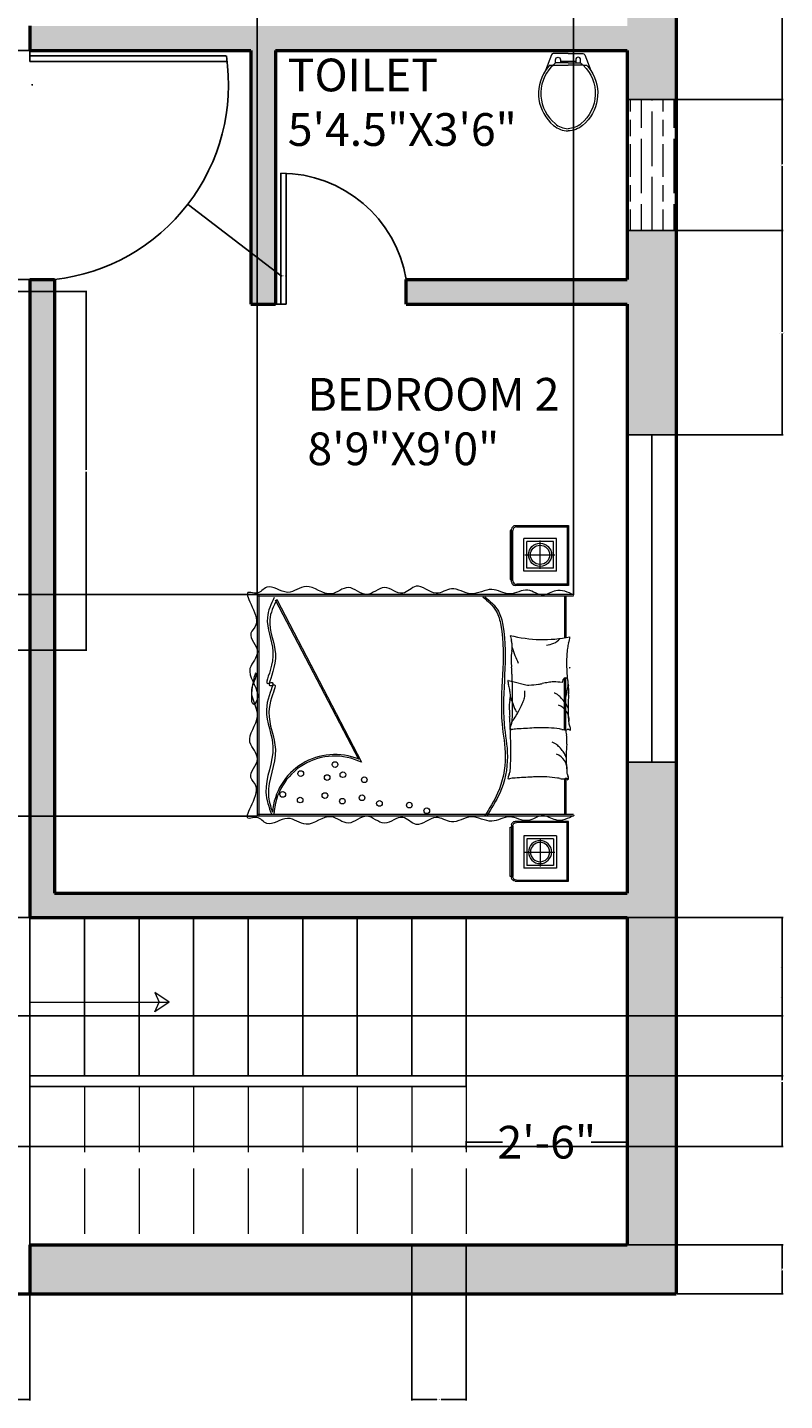
# Model space of a CAD drawing. Units: inches. Extents: x -2 to 282, y -370 to 35.
# Tile 3 of 5: x 143 to 282, y -370 to -119. Entities that reach past the tile are written whole.
import ezdxf

# ---------------------------------------------------------------- set-up
doc = ezdxf.new("R2010")
doc.units = ezdxf.units.IN
doc.header["$MEASUREMENT"] = 0
doc.linetypes.add('ACAD_ISO02W100', pattern=[15, 12, -3])
for name, color, linetype, lineweight in [('A-ANNO-DIMS', 2, 'Continuous', 18), ('A-ANNO-SYMB', 7, 'Continuous', 18), ('A-AREA-IDEN', 7, 'Continuous', 25), ('A-DOOR', 3, 'Continuous', 25), ('A-FLOR-FIXT', 9, 'Continuous', 18), ('A-FLOR-STRS', 7, 'Continuous', 25), ('A-FLOR-STRS-OVHD', 8, 'ACAD_ISO02W100', 18), ('A-FURN', 8, 'Continuous', 18), ('A-GLAZ', 4, 'Continuous', 25), ('A-GLAZ-PATT', 9, 'Continuous', 13), ('A-WALL', 7, 'Continuous', 50), ('A-WALL-PATT', 252, 'Continuous', 13)]:
    doc.layers.add(name, color=color, linetype=linetype, lineweight=lineweight)
doc.styles.get("Standard").update_dxf_attribs({"font": 'arial.ttf'})
doc.dimstyles.get("Standard").update_dxf_attribs({"dimtxt": 0.18, "dimasz": 0.18, "dimexe": 0.18, "dimexo": 0.0625, "dimgap": 0.09, "dimtad": 0, "dimtih": 1, "dimtoh": 1, "dimdec": 0, "dimzin": 0, "dimdsep": 46, "dimlunit": 3, "dimtxsty": 'Standard', "dimcen": 0.09, "dimadec": 0, "dimazin": 0, "dimtfac": 1, "dimtdec": 0, "dimtofl": 0, "dimtmove": 0, "dimatfit": 3, "dimfxl": 1, "dimtolj": 1, "dimtzin": 0, "dimarcsym": 0})

# ---------------------------------------------------------------- blocks, each defined once
blk = doc.blocks.new('*D1')
at = {"layer": 'A-ANNO-DIMS', "color": 0, "lineweight": -2, "transparency": 16777216}
for p, q in [((223.91, -324.22), (223.91, -322.81)), ((224.09, -322.99), (230.55, -322.99)), ((253.23, -322.99), (246.78, -322.99)), ((253.41, -324.22), (253.41, -322.81))]:
    blk.add_line(p, q, dxfattribs=at)
at = {"layer": 'A-ANNO-DIMS', "color": 0, "transparency": 16777216}
for points in [[(224.09, -322.96), (224.09, -323.02), (223.91, -322.99)], [(253.23, -322.96), (253.23, -323.02), (253.41, -322.99)]]:
    blk.add_solid(points, dxfattribs=at)
at = {"layer": 'Defpoints', "color": 0, "transparency": 16777216}
for p in [(223.91, -324.28), (253.41, -322.99), (253.41, -324.28)]:
    blk.add_point(p, dxfattribs=at)
at = {"layer": 'A-ANNO-DIMS', "color": 0, "transparency": 16777216, "insert": (238.66, -322.99), "char_height": 6, "attachment_point": 5}
blk.add_mtext('\\A1;2\'-6"', dxfattribs=at)
blk = doc.blocks.new('WINDOW-60IN')
for p, q in [((0, 0), (0, 60)), ((0, 60), (9, 60)), ((4.5, 60), (4.5, 0)), ((9, 60), (9, 0)), ((9, 0), (0, 0))]:
    blk.add_line(p, q)
blk = doc.blocks.new('DOOR-SWING-24IN')
for p, q in [((24, 2), (0, 2)), ((24, 1), (0, 1)), ((24, 0), (24, 2))]:
    blk.add_line(p, q)
blk.add_arc((23.32, 1), 23.31, 99.4157, 180)
blk = doc.blocks.new('WC-PLAN')
for p, q in [((2.03, 12.04), (2.63, 12.04)), ((2.63, 12.04), (5.42, 12.04)), ((8.21, 12.04), (5.42, 12.04)), ((8.21, 12.04), (8.81, 12.04))]:
    blk.add_line(p, q)
for points in [[(5.42, 14.19), (2.71, 14.19, 0.31031), (2.38, 13.97), (1.26, 11.07, 0.209071)], [(3.12, 12.47), (3.12, 13.07, -1), (4.02, 13.07), (4.02, 12.76)], [(5.42, 14.19), (8.13, 14.19, -0.31031), (8.46, 13.97), (9.58, 11.07, -0.209071)], [(7.72, 12.47), (7.72, 13.07, 1), (6.82, 13.07), (6.82, 12.76)], [(1.26, 11.07, 0.383919), (2.75, 1.02, 0.163732), (5.42, 0, 0.359733)], [(2.34, 11.76, 0.431639), (3.02, 1.35, 0.162618), (5.42, 0.42, 0.470877)], [(2.03, 12.04, 0.040937), (1.26, 11.07, 0.163732)], [(2.63, 12.04, 0.014165), (2.34, 11.76, 0.162618)], [(3.12, 12.47, 0.022712), (2.63, 12.04, 0.162618)], [(5.42, 12.47), (3.12, 12.47, 0.022712)], [(5.42, 12.47), (7.72, 12.47, -0.476108)], [(8.21, 12.04, -0.448546), (7.82, 1.35, -0.162618), (5.42, 0.42, -0.470877)], [(9.58, 11.07, -0.383919), (8.09, 1.02, -0.163732), (5.42, 0, -0.359733)], [(7.72, 12.47, -0.022712), (8.21, 12.04, -0.162618)], [(8.81, 12.04, -0.040937), (9.58, 11.07, -0.163732)]]:
    blk.add_lwpolyline(points, format="xyb")
for points in [[(6.82, 12.76), (4.02, 12.76)], [(4.02, 12.76), (4.02, 12.47)], [(6.82, 12.76), (6.82, 12.47)]]:
    blk.add_lwpolyline(points)
blk = doc.blocks.new('BEDSIDE-TABLE')
for p, q in [((0, 0.94), (0, 10.72)), ((0, 10.72), (11.02, 10.72)), ((0, 10.5), (11.02, 10.5)), ((0.22, 1.16), (0.22, 10.72)), ((10.8, 10.72), (10.8, 1.16)), ((11.02, 10.72), (11.02, 0.94)), ((2.39, 8.51), (2.39, 2.55)), ((8.35, 8.51), (2.39, 8.51)), ((2.92, 7.98), (2.92, 3.08)), ((7.82, 7.98), (2.92, 7.98)), ((5.37, 2.73), (5.37, 8.22)), ((7.82, 7.98), (7.82, 3.08)), ((8.35, 8.51), (8.35, 2.55)), ((7.94, 5.51), (2.73, 5.51)), ((8.35, 2.55), (2.39, 2.55)), ((7.82, 3.08), (2.92, 3.08)), ((10.37, 0.28), (0.66, 0.28)), ((10.15, 0.5), (0.87, 0.5))]:
    blk.add_line(p, q)
blk.add_lwpolyline([(9.94, 0.26), (0.88, 0.26), (0.88, 0), (9.94, 0)], close=True)
for radius in [2.13, 1.77]:
    blk.add_circle((5.37, 5.51), radius)
for centre, start, end in [((0.66, 0.94), 180, 270), ((0.87, 1.16), 180, 270), ((10.15, 1.16), 270, 0), ((10.37, 0.94), 270, 0)]:
    blk.add_arc(centre, 0.655, start, end)
blk = doc.blocks.new('*D26')
at = {"layer": 'A-ANNO-DIMS', "color": 0, "lineweight": -2, "transparency": 16777216}
for p, q in [((262.48, -89.06), (281.97, -89.06)), ((281.79, -89.24), (281.79, -110.25)), ((281.79, -131.63), (281.79, -110.62)), ((262.48, -131.81), (281.97, -131.81))]:
    blk.add_line(p, q, dxfattribs=at)
at = {"layer": 'A-ANNO-DIMS', "color": 0, "transparency": 16777216}
for points in [[(281.76, -89.24), (281.82, -89.24), (281.79, -89.06)], [(281.76, -131.63), (281.82, -131.63), (281.79, -131.81)]]:
    blk.add_solid(points, dxfattribs=at)
at = {"layer": 'Defpoints', "color": 0, "transparency": 16777216}
for p in [(262.41, -89.06), (262.41, -131.81), (281.79, -131.81)]:
    blk.add_point(p, dxfattribs=at)
at = {"layer": 'A-ANNO-DIMS', "color": 0, "transparency": 16777216, "insert": (281.79, -110.44), "char_height": 0.18, "attachment_point": 5}
blk.add_mtext('\\A1;3\'-7"', dxfattribs=at)
blk = doc.blocks.new('*D27')
at = {"layer": 'A-ANNO-DIMS', "color": 0, "lineweight": -2, "transparency": 16777216}
for p, q in [((262.48, -131.81), (281.97, -131.81)), ((281.79, -131.99), (281.79, -143.63)), ((281.79, -155.63), (281.79, -143.99)), ((262.48, -155.81), (281.97, -155.81))]:
    blk.add_line(p, q, dxfattribs=at)
at = {"layer": 'A-ANNO-DIMS', "color": 0, "transparency": 16777216}
for points in [[(281.76, -131.99), (281.82, -131.99), (281.79, -131.81)], [(281.76, -155.63), (281.82, -155.63), (281.79, -155.81)]]:
    blk.add_solid(points, dxfattribs=at)
at = {"layer": 'Defpoints', "color": 0, "transparency": 16777216}
for p in [(262.41, -131.81), (262.41, -155.81), (281.79, -155.81)]:
    blk.add_point(p, dxfattribs=at)
at = {"layer": 'A-ANNO-DIMS', "color": 0, "transparency": 16777216, "insert": (281.79, -143.81), "char_height": 0.18, "attachment_point": 5}
blk.add_mtext('\\A1;2\'-0"', dxfattribs=at)
blk = doc.blocks.new('*D28')
at = {"layer": 'A-ANNO-DIMS', "color": 0, "lineweight": -2, "transparency": 16777216}
for p, q in [((262.48, -155.81), (281.97, -155.81)), ((281.79, -155.99), (281.79, -174.38)), ((281.79, -193.13), (281.79, -174.74)), ((262.48, -193.31), (281.97, -193.31))]:
    blk.add_line(p, q, dxfattribs=at)
at = {"layer": 'A-ANNO-DIMS', "color": 0, "transparency": 16777216}
for points in [[(281.76, -155.99), (281.82, -155.99), (281.79, -155.81)], [(281.76, -193.13), (281.82, -193.13), (281.79, -193.31)]]:
    blk.add_solid(points, dxfattribs=at)
at = {"layer": 'Defpoints', "color": 0, "transparency": 16777216}
for p in [(262.41, -155.81), (262.41, -193.31), (281.79, -193.31)]:
    blk.add_point(p, dxfattribs=at)
at = {"layer": 'A-ANNO-DIMS', "color": 0, "transparency": 16777216, "insert": (281.79, -174.56), "char_height": 0.18, "attachment_point": 5}
blk.add_mtext('\\A1;3\'-1 1/2"', dxfattribs=at)
blk = doc.blocks.new('*D31')
at = {"layer": 'A-ANNO-DIMS', "color": 0, "lineweight": -2, "transparency": 16777216}
for p, q in [((31.48, -281.81), (281.97, -281.81)), ((281.79, -281.99), (281.79, -290.63)), ((281.79, -299.63), (281.79, -290.99)), ((31.48, -299.81), (281.97, -299.81))]:
    blk.add_line(p, q, dxfattribs=at)
at = {"layer": 'A-ANNO-DIMS', "color": 0, "transparency": 16777216}
for points in [[(281.76, -281.99), (281.82, -281.99), (281.79, -281.81)], [(281.76, -299.63), (281.82, -299.63), (281.79, -299.81)]]:
    blk.add_solid(points, dxfattribs=at)
at = {"layer": 'Defpoints', "color": 0, "transparency": 16777216}
for p in [(31.41, -281.81), (31.41, -299.81), (281.79, -299.81)]:
    blk.add_point(p, dxfattribs=at)
at = {"layer": 'A-ANNO-DIMS', "color": 0, "transparency": 16777216, "insert": (281.79, -290.81), "char_height": 0.18, "attachment_point": 5}
blk.add_mtext('\\A1;1\'-6"', dxfattribs=at)
blk = doc.blocks.new('*D32')
at = {"layer": 'A-ANNO-DIMS', "color": 0, "lineweight": -2, "transparency": 16777216}
for p, q in [((31.48, -299.81), (281.97, -299.81)), ((281.79, -299.99), (281.79, -311.63)), ((281.79, -323.63), (281.79, -311.99)), ((31.48, -323.81), (281.97, -323.81))]:
    blk.add_line(p, q, dxfattribs=at)
at = {"layer": 'A-ANNO-DIMS', "color": 0, "transparency": 16777216}
for points in [[(281.76, -299.99), (281.82, -299.99), (281.79, -299.81)], [(281.76, -323.63), (281.82, -323.63), (281.79, -323.81)]]:
    blk.add_solid(points, dxfattribs=at)
at = {"layer": 'Defpoints', "color": 0, "transparency": 16777216}
for p in [(31.41, -299.81), (31.41, -323.81), (281.79, -323.81)]:
    blk.add_point(p, dxfattribs=at)
at = {"layer": 'A-ANNO-DIMS', "color": 0, "transparency": 16777216, "insert": (281.79, -311.81), "char_height": 0.18, "attachment_point": 5}
blk.add_mtext('\\A1;2\'-0"', dxfattribs=at)
blk = doc.blocks.new('*D36')
at = {"layer": 'A-ANNO-DIMS', "color": 0, "lineweight": -2, "transparency": 16777216}
for p, q in [((107.91, -281.87), (107.91, -370.37)), ((143.91, -281.87), (143.91, -370.37)), ((108.09, -370.19), (125.58, -370.19)), ((143.73, -370.19), (126.24, -370.19))]:
    blk.add_line(p, q, dxfattribs=at)
at = {"layer": 'A-ANNO-DIMS', "color": 0, "transparency": 16777216}
for points in [[(108.09, -370.16), (108.09, -370.22), (107.91, -370.19)], [(143.73, -370.16), (143.73, -370.22), (143.91, -370.19)]]:
    blk.add_solid(points, dxfattribs=at)
at = {"layer": 'Defpoints', "color": 0, "transparency": 16777216}
for p in [(107.91, -281.81), (143.91, -281.81), (143.91, -370.19)]:
    blk.add_point(p, dxfattribs=at)
at = {"layer": 'A-ANNO-DIMS', "color": 0, "transparency": 16777216, "insert": (125.91, -370.19), "char_height": 0.18, "attachment_point": 5}
blk.add_mtext('\\A1;3\'-0"', dxfattribs=at)
blk = doc.blocks.new('*D40')
at = {"layer": 'A-ANNO-DIMS', "color": 0, "lineweight": -2, "transparency": 16777216}
for p, q in [((213.91, -341.87), (213.91, -370.37)), ((223.91, -341.87), (223.91, -370.37)), ((214.09, -370.19), (218.51, -370.19)), ((223.73, -370.19), (219.31, -370.19))]:
    blk.add_line(p, q, dxfattribs=at)
at = {"layer": 'A-ANNO-DIMS', "color": 0, "transparency": 16777216}
for points in [[(214.09, -370.16), (214.09, -370.22), (213.91, -370.19)], [(223.73, -370.16), (223.73, -370.22), (223.91, -370.19)]]:
    blk.add_solid(points, dxfattribs=at)
at = {"layer": 'Defpoints', "color": 0, "transparency": 16777216}
for p in [(213.91, -341.81), (223.91, -341.81), (223.91, -370.19)]:
    blk.add_point(p, dxfattribs=at)
at = {"layer": 'A-ANNO-DIMS', "color": 0, "transparency": 16777216, "insert": (218.91, -370.19), "char_height": 0.18, "attachment_point": 5}
blk.add_mtext('\\A1;0\'-10"', dxfattribs=at)
blk = doc.blocks.new('*D41')
at = {"layer": 'A-ANNO-DIMS', "color": 0, "lineweight": -2, "transparency": 16777216}
for p, q in [((223.98, -281.81), (281.97, -281.81)), ((281.79, -281.99), (281.79, -296.13)), ((281.79, -310.63), (281.79, -296.49)), ((223.98, -310.81), (281.97, -310.81))]:
    blk.add_line(p, q, dxfattribs=at)
at = {"layer": 'A-ANNO-DIMS', "color": 0, "transparency": 16777216}
for points in [[(281.76, -281.99), (281.82, -281.99), (281.79, -281.81)], [(281.76, -310.63), (281.82, -310.63), (281.79, -310.81)]]:
    blk.add_solid(points, dxfattribs=at)
at = {"layer": 'Defpoints', "color": 0, "transparency": 16777216}
for p in [(223.91, -281.81), (223.91, -310.81), (281.79, -310.81)]:
    blk.add_point(p, dxfattribs=at)
at = {"layer": 'A-ANNO-DIMS', "color": 0, "transparency": 16777216, "insert": (281.79, -296.31), "char_height": 0.18, "attachment_point": 5}
blk.add_mtext('\\A1;2\'-5"', dxfattribs=at)
blk = doc.blocks.new('*D44')
at = {"layer": 'A-ANNO-DIMS', "color": 0, "lineweight": -2, "transparency": 16777216}
for p, q in [((253.48, -341.81), (281.97, -341.81)), ((281.79, -341.99), (281.79, -346.13)), ((281.79, -350.63), (281.79, -346.49)), ((262.48, -350.81), (281.97, -350.81))]:
    blk.add_line(p, q, dxfattribs=at)
at = {"layer": 'A-ANNO-DIMS', "color": 0, "transparency": 16777216}
for points in [[(281.76, -341.99), (281.82, -341.99), (281.79, -341.81)], [(281.76, -350.63), (281.82, -350.63), (281.79, -350.81)]]:
    blk.add_solid(points, dxfattribs=at)
at = {"layer": 'Defpoints', "color": 0, "transparency": 16777216}
for p in [(253.41, -341.81), (262.41, -350.81), (281.79, -350.81)]:
    blk.add_point(p, dxfattribs=at)
at = {"layer": 'A-ANNO-DIMS', "color": 0, "transparency": 16777216, "insert": (281.79, -346.31), "char_height": 0.18, "attachment_point": 5}
blk.add_mtext('\\A1;0\'-9"', dxfattribs=at)
blk = doc.blocks.new('*D49')
at = {"layer": 'A-ANNO-DIMS', "color": 0, "lineweight": -2, "transparency": 16777216}
for p, q in [((134.88, -166.98), (154.37, -166.98)), ((154.19, -167.16), (154.19, -199.71)), ((154.19, -232.61), (154.19, -200.07)), ((134.88, -232.79), (154.37, -232.79))]:
    blk.add_line(p, q, dxfattribs=at)
at = {"layer": 'A-ANNO-DIMS', "color": 0, "transparency": 16777216}
for points in [[(154.16, -167.16), (154.22, -167.16), (154.19, -166.98)], [(154.16, -232.61), (154.22, -232.61), (154.19, -232.79)]]:
    blk.add_solid(points, dxfattribs=at)
at = {"layer": 'Defpoints', "color": 0, "transparency": 16777216}
for p in [(134.81, -166.98), (134.81, -232.79), (154.19, -232.79)]:
    blk.add_point(p, dxfattribs=at)
at = {"layer": 'A-ANNO-DIMS', "color": 0, "transparency": 16777216, "insert": (154.19, -199.89), "char_height": 0.18, "attachment_point": 5}
blk.add_mtext('\\A1;5\'-6"', dxfattribs=at)
blk = doc.blocks.new('*D52')
at = {"layer": 'A-ANNO-DIMS', "color": 0, "lineweight": -2, "transparency": 16777216}
for p, q in [((185.58, -222.52), (185.58, 28.74)), ((185.76, 28.56), (214.16, 28.56)), ((243.38, 28.56), (214.97, 28.56)), ((243.56, -222.52), (243.56, 28.74))]:
    blk.add_line(p, q, dxfattribs=at)
at = {"layer": 'A-ANNO-DIMS', "color": 0, "transparency": 16777216}
for points in [[(185.76, 28.59), (185.76, 28.53), (185.58, 28.56)], [(243.38, 28.59), (243.38, 28.53), (243.56, 28.56)]]:
    blk.add_solid(points, dxfattribs=at)
at = {"layer": 'Defpoints', "color": 0, "transparency": 16777216}
for p in [(243.56, 28.56), (185.58, -222.58), (243.56, -222.58)]:
    blk.add_point(p, dxfattribs=at)
at = {"layer": 'A-ANNO-DIMS', "color": 0, "transparency": 16777216, "insert": (214.57, 28.56), "char_height": 0.18, "attachment_point": 5}
blk.add_mtext('\\A1;4\'-10"', dxfattribs=at)
blk = doc.blocks.new('*D53')
at = {"layer": 'A-ANNO-DIMS', "color": 0, "lineweight": -2, "transparency": 16777216}
for p, q in [((185.51, -222.58), (2.86, -222.58)), ((3.04, -222.76), (3.04, -242.71)), ((3.04, -263.02), (3.04, -243.07)), ((185.51, -263.2), (2.86, -263.2))]:
    blk.add_line(p, q, dxfattribs=at)
at = {"layer": 'A-ANNO-DIMS', "color": 0, "transparency": 16777216}
for points in [[(3.01, -222.76), (3.07, -222.76), (3.04, -222.58)], [(3.01, -263.02), (3.07, -263.02), (3.04, -263.2)]]:
    blk.add_solid(points, dxfattribs=at)
at = {"layer": 'Defpoints', "color": 0, "transparency": 16777216}
for p in [(3.04, -222.58), (185.58, -222.58), (185.58, -263.2)]:
    blk.add_point(p, dxfattribs=at)
at = {"layer": 'A-ANNO-DIMS', "color": 0, "transparency": 16777216, "insert": (3.04, -242.89), "char_height": 0.18, "attachment_point": 5}
blk.add_mtext('\\A1;3\'-4 1/2"', dxfattribs=at)
blk = doc.blocks.new('*D59')
at = {"layer": 'A-ANNO-DIMS', "color": 0, "lineweight": -2, "transparency": 16777216}
for p, q in [((143.85, -122.81), (124.36, -122.81)), ((124.54, -122.99), (124.54, -143.63)), ((124.54, -164.63), (124.54, -143.99)), ((143.85, -164.81), (124.36, -164.81))]:
    blk.add_line(p, q, dxfattribs=at)
at = {"layer": 'A-ANNO-DIMS', "color": 0, "transparency": 16777216}
for points in [[(124.51, -122.99), (124.57, -122.99), (124.54, -122.81)], [(124.51, -164.63), (124.57, -164.63), (124.54, -164.81)]]:
    blk.add_solid(points, dxfattribs=at)
at = {"layer": 'Defpoints', "color": 0, "transparency": 16777216}
for p in [(124.54, -122.81), (143.91, -122.81), (143.91, -164.81)]:
    blk.add_point(p, dxfattribs=at)
at = {"layer": 'A-ANNO-DIMS', "color": 0, "transparency": 16777216, "insert": (124.54, -143.81), "char_height": 0.18, "attachment_point": 5}
blk.add_mtext('\\A1;3\'-6"', dxfattribs=at)
blk = doc.blocks.new('*D61')
at = {"layer": 'A-ANNO-DIMS', "color": 0, "lineweight": -2, "transparency": 16777216}
for p, q in [((144.26, -129.08), (144.44, -129.08)), ((144.35, -129.17), (144.35, -128.99)), ((189.97, -164.13), (173, -151.1)), ((190.15, -164.13), (189.97, -164.13))]:
    blk.add_line(p, q, dxfattribs=at)
at = {"layer": 'A-ANNO-DIMS', "color": 0, "transparency": 16777216}
blk.add_solid([(173.02, -151.08), (172.98, -151.12), (172.86, -150.99)], dxfattribs=at)
at = {"layer": 'Defpoints', "color": 0, "transparency": 16777216}
for p in [(144.35, -129.08), (172.86, -150.99)]:
    blk.add_point(p, dxfattribs=at)
at = {"layer": 'A-ANNO-DIMS', "color": 0, "transparency": 16777216, "insert": (190.56, -164.13), "char_height": 0.18, "attachment_point": 5}
blk.add_mtext('\\A1;R3\'-0"', dxfattribs=at)

msp = doc.modelspace()

# ---------------------------------------------------------------- hatches: boundary and pattern name
at = {"layer": 'A-GLAZ-PATT'}
h = msp.add_hatch(dxfattribs=at)
h.set_pattern_fill('GOST_WOOD', color=256)
h.set_pattern_definition([(90, (0, 0), (6, -4e-16), [10, -2]), (90, (2, -2), (6, -4e-16), [6, -1.5, 3, -1.5]), (90, (4, -5), (6, -4e-16), [10, -2])])
h.paths.add_polyline_path([(134.91, 9.19), (110.91, 9.19), (110.91, 0.19), (134.91, 0.19)])
h.paths.add_polyline_path([(262.41, -131.81), (253.41, -131.81), (253.41, -155.81), (262.41, -155.81)])
at = {"layer": 'A-WALL-PATT'}
h = msp.add_hatch(color=256, dxfattribs=at)
h.dxf.hatch_style = 1
h.paths.add_polyline_path([(262.41, 9.19), (134.91, 9.19), (134.91, 0.19), (143.91, 0.19), (143.91, -35.81), (148.41, -35.81), (148.41, 0.19), (253.41, 0.19), (253.41, -29.06), (262.41, -29.06)])
h.paths.add_polyline_path([(110.91, 9.19), (22.41, 9.19), (22.41, -11.81), (31.41, -11.81), (31.41, 0.19), (97.41, 0.19), (97.41, -88.31), (101.91, -88.31), (101.91, -64.31), (143.91, -64.31), (143.91, -88.31), (148.41, -88.31), (148.41, -59.81), (101.91, -59.81), (101.91, 0.19), (110.91, 0.19)])
h.paths.add_polyline_path([(31.41, -88.31), (64.41, -88.31), (64.41, -83.81), (31.41, -83.81), (31.41, -71.81), (22.41, -71.81), (22.41, -121.2), (31.41, -121.2)])
h.paths.add_polyline_path([(262.41, -89.06), (253.41, -89.06), (253.41, -118.31), (143.91, -118.31), (143.91, -122.81), (184.41, -122.81), (184.41, -164.81), (184.41, -169.31), (188.91, -169.31), (188.91, -164.81), (188.91, -122.81), (253.41, -122.81), (253.41, -131.81), (262.41, -131.81)])
h.paths.add_polyline_path([(262.41, -155.81), (253.41, -155.81), (253.41, -164.81), (212.91, -164.81), (212.91, -169.31), (253.41, -169.31), (253.41, -193.31), (262.41, -193.31)])
h.paths.add_polyline_path([(262.41, -253.31), (253.41, -253.31), (253.41, -277.31), (148.41, -277.31), (148.41, -164.81), (143.91, -164.81), (143.91, -169.31), (143.91, -281.81), (253.41, -281.81), (253.41, -341.81), (143.91, -341.81), (143.91, -350.81), (262.41, -350.81)])
h.paths.add_polyline_path([(31.41, -323.81), (22.41, -323.81), (22.41, -350.81), (95.91, -350.81), (95.91, -281.81), (107.91, -281.81), (107.91, -277.31), (67.41, -277.31), (67.41, -281.81), (91.41, -281.81), (91.41, -341.81), (31.41, -341.81)])
h.paths.add_polyline_path([(43.41, -277.31), (31.41, -277.31), (31.41, -181.2), (22.41, -181.2), (22.41, -299.81), (31.41, -299.81), (31.41, -281.81), (43.41, -281.81)])

# ---------------------------------------------------------------- linework, layer by layer
at = {"layer": 'A-ANNO-SYMB'}
for p, q in [((169.41, -297.31), (166.82, -295.54)), ((166.82, -295.54), (167.63, -297.31)), ((143.91, -297.31), (169.41, -297.31)), ((169.41, -297.31), (166.82, -299.08)), ((166.82, -299.08), (167.63, -297.31))]:
    msp.add_line(p, q, dxfattribs=at)
at = {"layer": 'A-DOOR'}
for p, q in [((143.91, -122.81), (143.91, -124.81)), ((143.91, -123.81), (179.91, -123.81)), ((143.91, -124.81), (179.91, -124.81)), ((143.91, -281.81), (142.91, -281.81))]:
    msp.add_line(p, q, dxfattribs=at)
msp.add_arc((144.35, -129.08), 35.96, 276.4952, 8.4352, dxfattribs=at)
at = {"layer": 'A-FLOR-STRS'}
for p, q in [((143.91, -281.81), (143.91, -312.81)), ((153.91, -281.81), (153.91, -310.81)), ((163.91, -281.81), (163.91, -310.81)), ((173.91, -281.81), (173.91, -310.81)), ((183.91, -281.81), (183.91, -310.81)), ((193.91, -281.81), (193.91, -310.81)), ((203.91, -281.81), (203.91, -310.81)), ((213.91, -281.81), (213.91, -310.81)), ((223.91, -281.81), (223.91, -312.81)), ((143.91, -310.81), (223.91, -310.81)), ((143.91, -312.81), (223.91, -312.81))]:
    msp.add_line(p, q, dxfattribs=at)
at = {"layer": 'A-FLOR-STRS-OVHD'}
for p, q in [((143.91, -312.81), (143.91, -341.81)), ((153.91, -312.81), (153.91, -341.81)), ((163.91, -312.81), (163.91, -341.81)), ((173.91, -312.81), (173.91, -341.81)), ((183.91, -312.81), (183.91, -341.81)), ((193.91, -312.81), (193.91, -341.81)), ((203.91, -312.81), (203.91, -341.81)), ((213.91, -312.81), (213.91, -341.81)), ((223.91, -312.81), (223.91, -341.81))]:
    msp.add_line(p, q, dxfattribs=at)
at = {"layer": 'A-FURN'}
for p, q in [((185.58, -222.58), (185.58, -263.2)), ((243.56, -222.58), (185.58, -222.58)), ((243.56, -222.87), (185.58, -222.87)), ((185.87, -222.58), (185.87, -263.2)), ((188.89, -223.56), (204.17, -252.78)), ((189.17, -223.46), (204.69, -253.33)), ((241.89, -222.87), (241.89, -230.52)), ((242.18, -222.87), (242.18, -230.47)), ((231.56, -238.31), (232.43, -238.52)), ((232.43, -238.52), (234.83, -239.12)), ((241.89, -247.38), (241.89, -237.95)), ((242.18, -247.38), (242.18, -237.84)), ((241.89, -256.37), (241.89, -262.91)), ((242.18, -256.3), (242.18, -262.91)), ((243.56, -262.91), (185.58, -262.91)), ((243.56, -263.2), (185.58, -263.2))]:
    msp.add_line(p, q, dxfattribs=at)
for centre in [(199.85, -253.75), (193.56, -255.4), (198.4, -256.13), (201.29, -255.61), (205.21, -256.54), (190.26, -259.22), (197.99, -259.43), (204.8, -259.84), (193.45, -260.25), (201.19, -260.46), (207.99, -260.87), (213.46, -261.18), (216.66, -262.22)]:
    msp.add_circle(centre, 0.516, dxfattribs=at)
for centre, radius, start, end in [((238.04, -205.78), 25.04, 255.9578, 281.1903), ((238.53, -228.97), 6.66, 189.4841, 197.3864), ((228.86, -232), 3.47, 6.4341, 17.3864), ((228.11, -232.09), 4.23, 348.4414, 6.4341), ((238.2, -227.83), 4.06, 275.6311, 315.0976), ((249.42, -233.35), 7.02, 164.256, 172.4531), ((234.16, -229.05), 8.84, 344.256, 351.5628), ((238.79, -234.27), 6.67, 168.4414, 182.7491), ((252.79, -225.98), 21.41, 197.1982, 205.3111), ((262.08, -235.03), 19.79, 172.4531, 180), ((272.8, -232.64), 40.72, 182.7491, 184.6176), ((197.06, -238.75), 35.26, 2.6096, 4.6176), ((272.7, -235.03), 30.41, 180, 186.0867), ((242.87, -235.92), 0.0672, 168.1069, 289.564), ((242.86, -235.89), 0.0991, 289.564, 338.2117), ((231.56, -238.33), 0.0266, 75.9551, 184.0829), ((239.36, -237.78), 7.85, 184.0829, 189.4841), ((238.18, -237.97), 6.66, 189.4841, 197.3864), ((134.92, -241.59), 97.47, 0.9704, 2.6096), ((235.3, -237.22), 1.96, 255.9548, 272.6649), ((234.51, -220.1), 19.1, 272.6649, 278.0051), ((235.89, -229.91), 9.19, 278.0051, 282.1984), ((243.23, -263.89), 25.57, 99.6844, 102.1984), ((239.92, -244.51), 5.91, 90, 99.6844), ((239.92, -252.86), 14.26, 83.7676, 90), ((242.45, -238.76), 0.991, 116.5805, 175.5998), ((242.18, -238.22), 0.38, 11.2724, 116.5805), ((257.72, -236.62), 15.34, 186.0867, 190.1899), ((239.98, -238.66), 2.62, 0, 11.2724), ((237.93, -238.66), 4.67, 351.5628, 0), ((228.52, -241), 3.47, 6.4341, 17.3864), ((227.76, -241.08), 4.23, 348.4414, 6.4341), ((252.44, -234.98), 21.41, 197.1982, 205.3111), ((66.62, -242.74), 165.78, 359.7135, 0.9704), ((232.95, -241.13), 1.68, 339.3257, 355.9172), ((226.76, -240.69), 7.89, 355.9172, 3.5552), ((237.75, -245.97), 5.8, 61.6832, 66.9972), ((239.82, -242.12), 1.43, 50.9651, 61.6832), ((236.61, -246.08), 6.53, 43.8115, 50.9651), ((233.13, -249.42), 11.35, 38.3886, 43.8115), ((261.73, -244.02), 19.79, 172.4531, 180), ((249.07, -242.35), 7.02, 164.256, 172.4531), ((233.81, -238.05), 8.84, 344.256, 351.5628), ((267.88, -243.12), 25.31, 175.1982, 179.4243), ((238.27, -240.12), 4.42, 2.5386, 10.1899), ((234.29, -240.3), 8.4, 355.1982, 2.5386), ((238.44, -243.27), 6.67, 168.4414, 182.7491), ((272.46, -241.63), 40.72, 182.7491, 184.6176), ((198.65, -243.4), 33.74, 356.426, 359.7135), ((225.37, -239.96), 9.06, 327.865, 333.5015), ((196.33, -225.48), 41.52, 333.5015, 335.6735), ((220.78, -236.54), 14.69, 335.6735, 339.3257), ((239.87, -245.59), 2.88, 355.7841, 71.5603), ((272.35, -244.02), 30.41, 180, 186.0867), ((240.28, -243.76), 2.23, 27.2396, 38.3886), ((236.23, -245.84), 6.78, 20.8603, 27.2396), ((285.89, -243.3), 43.32, 179.4243, 181.9079), ((196.71, -247.75), 35.26, 2.6096, 4.6176), ((134.58, -250.58), 97.47, 0.9704, 2.6096), ((234.1, -247.51), 2.22, 152.7159, 163.7788), ((230.95, -245.89), 1.31, 332.7159, 347.131), ((228.11, -245.24), 4.23, 347.131, 356.426), ((215.16, -233.55), 21.12, 324.1737, 327.865), ((266.37, -243.95), 23.79, 181.9079, 185.2592), ((244.24, -245.99), 1.56, 185.2592, 210.6513), ((234.4, -247.6), 2.54, 163.7788, 172.8796), ((231.92, -247.29), 0.0383, 172.8796, 253.3022), ((232.07, -246.79), 0.56, 253.3022, 279.9984), ((66.28, -251.74), 165.78, 359.7135, 0.9704), ((233.78, -256.51), 9.31, 93.5049, 99.9984), ((257.38, -641.77), 395.29, 93.055, 93.5049), ((238.42, -286.56), 39.58, 91.6331, 93.055), ((237.85, -266.67), 19.68, 86.6313, 91.6331), ((237.45, -273.45), 26.47, 82.3191, 86.6313), ((240.22, -252.92), 5.75, 77.8905, 82.3191), ((242.93, -240.32), 7.13, 257.8905, 261.8665), ((242.05, -246.44), 0.951, 261.8665, 291.421), ((257.37, -245.62), 15.34, 186.0867, 190.1899), ((237.92, -249.12), 4.42, 2.5386, 10.1899), ((233.94, -249.29), 8.4, 355.1982, 2.5386), ((242.56, -247.75), 0.452, 68.0096, 111.421), ((242.69, -247.44), 0.124, 348.1069, 68.0096), ((242.17, -247.21), 0.837, 355.6975, 30.6513), ((242.28, -247.22), 0.728, 338.2117, 355.6975), ((237.4, -254.97), 5.8, 61.6832, 66.9972), ((239.47, -251.12), 1.43, 50.9651, 61.6832), ((236.26, -255.08), 6.53, 43.8115, 50.9651), ((232.78, -258.42), 11.35, 38.3886, 43.8115), ((239.94, -252.75), 2.23, 27.2396, 38.3886), ((235.88, -254.84), 6.78, 20.8603, 27.2396), ((267.54, -252.12), 25.31, 175.1982, 179.4243), ((199.79, -263.34), 11.44, 67.4442, 175.7493), ((199.79, -263.34), 11.15, 63.9063, 177.7674), ((198.31, -252.4), 33.74, 356.426, 359.7135), ((239.52, -254.59), 2.88, 355.7841, 71.5603), ((285.54, -252.3), 43.32, 179.4243, 181.9079), ((266.03, -252.95), 23.79, 181.9079, 185.2592), ((231.57, -256.29), 0.0383, 172.8796, 253.3022), ((234.05, -256.6), 2.54, 163.7788, 172.8796), ((231.72, -255.79), 0.56, 253.3022, 279.9984), ((233.75, -256.51), 2.22, 152.7159, 163.7788), ((230.61, -254.89), 1.31, 332.7159, 347.131), ((233.44, -265.51), 9.31, 93.5049, 99.9984), ((227.77, -254.24), 4.23, 347.131, 356.426), ((257.03, -650.77), 395.29, 93.055, 93.5049), ((238.08, -295.56), 39.58, 91.6331, 93.055), ((237.51, -275.67), 19.68, 86.6313, 91.6331), ((237.11, -282.45), 26.47, 82.3191, 86.6313), ((239.88, -261.92), 5.75, 77.8905, 82.3191), ((242.58, -249.32), 7.13, 257.8905, 261.8665), ((241.71, -255.44), 0.951, 261.8665, 291.421), ((242.22, -256.75), 0.452, 68.0096, 111.421), ((243.89, -254.99), 1.56, 185.2592, 210.6513), ((242.34, -256.44), 0.124, 348.1069, 68.0096), ((242.53, -256.48), 0.0672, 168.1069, 289.564), ((241.83, -256.21), 0.837, 355.6975, 30.6513), ((242.52, -256.45), 0.0991, 289.564, 338.2117), ((241.93, -256.22), 0.728, 338.2117, 355.6975)]:
    msp.add_arc(centre, radius, start, end, dxfattribs=at)
for points, knots in [([(243.66, -222.68), (242.53, -222.14), (240.59, -221.21), (237.83, -223.39), (235.06, -220.91), (231.85, -223.25), (228.43, -220.78), (224.82, -223.41), (221.43, -220.65), (218.08, -223.38), (214.97, -219.81), (212.1, -223.46), (208.86, -220.06), (205.64, -223.82), (202.36, -220.14), (198.72, -223.81), (194.89, -219.77), (191.12, -223.33), (187.66, -220.1), (185.88, -222.71), (181.9, -221.24), (187.05, -227.26), (183.41, -230.06), (186.94, -233.08), (182.77, -236.53), (187.02, -240.76), (183.67, -244.98), (185.23, -235.99), (185.52, -237.11)], [0, 0, 0, 0, 119.23822, 203.934156, 305.051348, 423.414205, 538.771408, 673.601551, 801.564672, 901.488314, 1036.739405, 1131.503109, 1252.869042, 1373.114912, 1497.089457, 1612.174498, 1779.078494, 1901.133447, 2037.052147, 2110.507177, 2158.377997, 2368.992723, 2430.676444, 2554.510696, 2670.523569, 2841.287389, 2999.108306, 3118.80064, 3118.80064, 3118.80064, 3118.80064]), ([(188.71, -223.1), (188.13, -224.31), (186.59, -227.49), (189.55, -233.26), (185.98, -240.85), (189.67, -236.86), (186.26, -244.15), (189.8, -251.01), (186.29, -257.51), (187.72, -261.56), (188.23, -262.91)], [0, 0, 0, 0, 134.096191, 351.943146, 593.51487, 936.925241, 1129.231545, 1368.385454, 1657.415202, 1803.02854, 1803.02854, 1803.02854, 1803.02854]), ([(189.16, -223.51), (188.57, -224.72), (187.04, -227.91), (190, -233.67), (186.42, -241.27), (190.11, -237.27), (186.71, -244.57), (190.24, -251.42), (186.89, -257.64), (187.99, -261.42), (188.38, -262.5)], [0, 0, 0, 0, 134.096191, 351.943146, 593.51487, 936.925241, 1129.231545, 1368.385454, 1657.415202, 1773.3935, 1773.3935, 1773.3935, 1773.3935]), ([(226.92, -223), (227.87, -223.79), (229.55, -225.18), (231.54, -233.35), (229.45, -242.32), (231.5, -252.54), (230.23, -258.53), (228.13, -261.81), (227.27, -263.16)], [0, 0, 0, 0, 3.597854, 6.329739, 24.437188, 30.418477, 37.31145, 42.080965, 42.080965, 42.080965, 42.080965]), ([(227.3, -223), (228.26, -223.79), (229.93, -225.18), (231.93, -233.35), (229.83, -242.32), (231.89, -252.54), (230.62, -258.53), (228.52, -261.81), (227.66, -263.16)], [0, 0, 0, 0, 3.597854, 6.329739, 24.437188, 30.418477, 37.31145, 42.080965, 42.080965, 42.080965, 42.080965]), ([(243.66, -263.1), (242.53, -263.64), (240.59, -264.57), (237.83, -262.39), (235.06, -264.87), (231.85, -262.53), (228.43, -265), (224.82, -262.37), (221.43, -265.13), (218.08, -262.4), (214.97, -265.97), (212.1, -262.32), (208.86, -265.72), (205.64, -261.96), (202.36, -265.64), (198.72, -261.96), (194.89, -266.01), (191.12, -262.45), (187.66, -265.68), (185.88, -263.07), (181.9, -264.54), (187.05, -258.52), (183.41, -255.72), (186.94, -252.7), (182.77, -249.25), (187.02, -245.02), (183.67, -240.8), (185.23, -238.23), (185.52, -237.11)], [0, 0, 0, 0, 119.23822, 203.934156, 305.051348, 423.414205, 538.771408, 673.601551, 801.564672, 901.488314, 1036.739405, 1131.503109, 1252.869042, 1373.114912, 1497.089457, 1612.174498, 1779.078494, 1901.133447, 2037.052147, 2110.507177, 2158.377997, 2368.992723, 2430.676444, 2554.510696, 2670.523569, 2841.287389, 2999.108306, 3118.80064, 3118.80064, 3118.80064, 3118.80064])]:
    msp.add_open_spline(points, degree=3, knots=knots, dxfattribs=at)
at = {"layer": 'A-GLAZ'}
for p, q in [((253.41, -155.81), (253.41, -131.81)), ((253.41, -131.81), (262.41, -131.81)), ((262.41, -131.81), (262.41, -155.81)), ((262.41, -155.81), (253.41, -155.81))]:
    msp.add_line(p, q, dxfattribs=at)
at = {"layer": 'A-WALL'}
for p, q in [((262.41, 9.19), (262.41, -350.81)), ((143.91, -118.31), (143.91, -122.81)), ((143.91, -122.81), (184.41, -122.81)), ((184.41, -122.81), (184.41, -164.81)), ((188.91, -122.81), (188.91, -164.81)), ((188.91, -122.81), (253.41, -122.81)), ((253.41, -122.81), (253.41, -164.81)), ((143.91, -164.81), (148.41, -164.81)), ((143.91, -164.81), (143.91, -169.31)), ((148.41, -164.81), (148.41, -277.31)), ((184.41, -164.81), (184.41, -169.31)), ((188.91, -164.81), (188.91, -169.31)), ((212.91, -169.31), (212.91, -164.81)), ((212.91, -164.81), (253.41, -164.81)), ((143.91, -169.31), (143.91, -281.81)), ((184.41, -169.31), (188.91, -169.31)), ((212.91, -169.31), (253.41, -169.31)), ((253.41, -169.31), (253.41, -277.31)), ((148.41, -277.31), (253.41, -277.31)), ((143.91, -281.81), (253.41, -281.81)), ((253.41, -281.81), (253.41, -341.81)), ((143.91, -341.81), (253.41, -341.81)), ((143.91, -341.81), (143.91, -350.81)), ((22.41, -350.81), (262.41, -350.81))]:
    msp.add_line(p, q, dxfattribs=at)

# ---------------------------------------------------------------- block references
at = {"layer": 'A-DOOR', "rotation": 270.0000000000003}
msp.add_blockref('DOOR-SWING-24IN', (188.91, -145.31), dxfattribs=at)
at = {"layer": 'A-FLOR-FIXT'}
msp.add_blockref('WC-PLAN', (237.15, -137.57), dxfattribs=at)
at = {"layer": 'A-FURN', "xscale": 0.9959614805337388, "yscale": 0.9959614805337388, "rotation": 269.9999999999993}
msp.add_blockref('BEDSIDE-TABLE', (231.94, -209.94), dxfattribs=at)
at = {"layer": 'A-FURN', "extrusion": (0, 0, -1), "xscale": 0.9959614805337388, "yscale": 0.9959614805337388, "zscale": -1, "rotation": 89.99999999754598}
msp.add_blockref('BEDSIDE-TABLE', (-231.94, -275.14), dxfattribs=at)
at = {"layer": 'A-GLAZ'}
msp.add_blockref('WINDOW-60IN', (253.41, -253.31), dxfattribs=at)

# ---------------------------------------------------------------- texts
at = {"layer": 'A-AREA-IDEN', "char_height": 6, "attachment_point": 1}
for s, insert in [('TOILET\\P5\'4.5"X3\'6"', (191.18, -124.3)), ('BEDROOM 2\\P8\'9"X9\'0"', (194.78, -182.85))]:
    msp.add_mtext(s, dxfattribs=dict(at, insert=insert))

# ---------------------------------------------------------------- dimensions: what is measured, and where the dimension line sits
at = {"layer": 'A-ANNO-DIMS'}
for base, p1, p2, override, picture, middle in [((243.56, 28.56), (185.58, -222.58), (243.56, -222.58), {"dimdec": 1, "dimlfac": 1, "dimrnd": 0, "dimzin": 1, "dimdsep": 46, "dimlunit": 4, "dimfrac": 2}, '*D52', (214.57, 28.56)), ((143.91, -370.19), (107.91, -281.81), (143.91, -281.81), {"dimdec": 1, "dimlfac": 1, "dimrnd": 0, "dimzin": 1, "dimdsep": 46, "dimlunit": 4, "dimfrac": 2}, '*D36', (125.91, -370.19)), ((253.41338597, -322.9852815), (223.91338597, -324.27851404), (253.41338597, -324.27851404), {"dimtxt": 6, "dimclrd": 0, "dimclre": 0, "dimclrt": 0}, '*D1', (238.66338597, -322.9852815)), ((223.91, -370.19), (213.91, -341.81), (223.91, -341.81), {"dimdec": 1, "dimlfac": 1, "dimrnd": 0, "dimzin": 1, "dimdsep": 46, "dimlunit": 4, "dimfrac": 2}, '*D40', (218.91, -370.19))]:
    dim = msp.add_linear_dim(base=base, p1=p1, p2=p2, dimstyle='Standard', override=override, dxfattribs=at)
    dim.commit()
    dim.dimension.update_dxf_attribs({"geometry": picture, "text_midpoint": middle})
for base, p1, p2, angle, picture, middle in [((281.788386, -131.8101), (262.413386, -89.0601), (262.413386, -131.8101), 90, '*D26', (281.788386, -110.4351)), ((124.54, -122.81), (143.91, -164.81), (143.91, -122.81), 90, '*D59', (124.54, -143.81)), ((281.79, -155.81), (262.41, -131.81), (262.41, -155.81), 90, '*D27', (281.79, -143.81)), ((281.79, -193.31), (262.41, -155.81), (262.41, -193.31), 90, '*D28', (281.79, -174.56)), ((154.19, -232.79), (134.81, -166.98), (134.81, -232.79), 270, '*D49', (154.19, -199.89)), ((3.04, -222.58), (185.58, -263.2), (185.58, -222.58), 90, '*D53', (3.04, -242.89)), ((281.79, -299.81), (31.41, -281.81), (31.41, -299.81), 90, '*D31', (281.79, -290.81)), ((281.79, -310.81), (223.91, -281.81), (223.91, -310.81), 90, '*D41', (281.79, -296.31)), ((281.79, -323.81), (31.41, -299.81), (31.41, -323.81), 90, '*D32', (281.79, -311.81)), ((281.79, -350.81), (253.41, -341.81), (262.41, -350.81), 90, '*D44', (281.79, -346.31))]:
    dim = msp.add_linear_dim(base=base, p1=p1, p2=p2, angle=angle, dimstyle='Standard', override={"dimdec": 1, "dimlfac": 1, "dimrnd": 0, "dimzin": 1, "dimdsep": 46, "dimlunit": 4, "dimfrac": 2}, dxfattribs=at)
    dim.commit()
    dim.dimension.update_dxf_attribs({"geometry": picture, "text_midpoint": middle})
dim = msp.add_radius_dim(center=(144.35, -129.08), mpoint=(172.86, -150.99), dimstyle='Standard', override={"dimdec": 1, "dimlfac": 1, "dimrnd": 0, "dimzin": 1, "dimdsep": 46, "dimlunit": 4, "dimfrac": 2}, dxfattribs=at)
dim.commit()
dim.dimension.update_dxf_attribs({"geometry": '*D61', "text_midpoint": (190.56, -164.13), "dimtype": 164})

doc.saveas('drawing.dxf')
